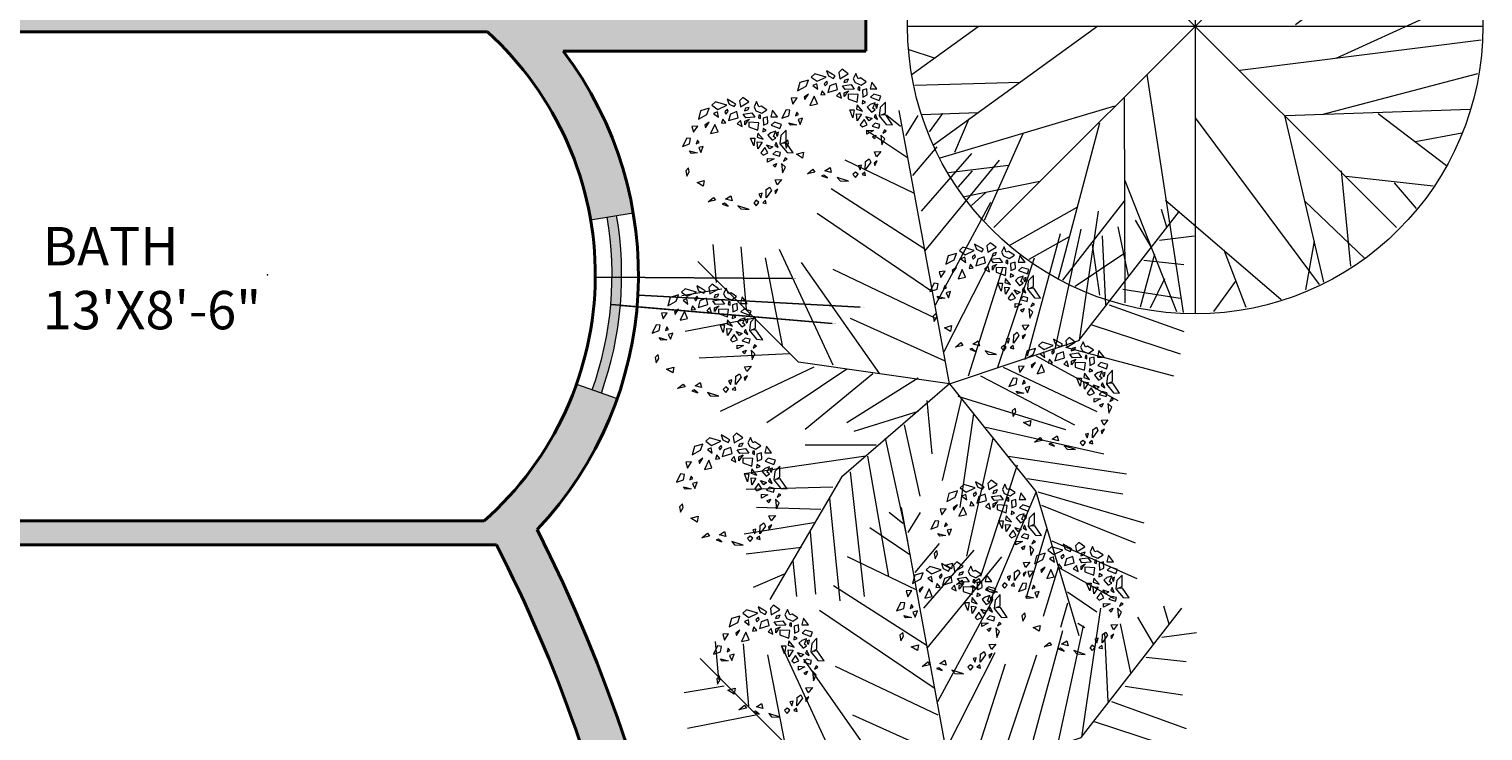
# Model space of a CAD drawing. Units: inches. Extents: x 2330 to 3943, y 1763 to 3461.
# Tile 30 of 40: x 3281 to 3584, y 2829 to 2975. Entities that reach past the tile are written whole.
import ezdxf

# ---------------------------------------------------------------- set-up
doc = ezdxf.new("R2010")
doc.units = ezdxf.units.IN
for name, color, linetype, lineweight in [('A-ANNO-DIMS', 2, 'Continuous', 18), ('A-AREA-IDEN', 7, 'Continuous', 18), ('A-GLAZ', 4, 'Continuous', 18), ('A-WALL', 7, 'Continuous', 40), ('A-WALL-PATT', 252, 'Continuous', 13), ('L-PLNT', 94, 'Continuous', 13)]:
    doc.layers.add(name, color=color, linetype=linetype, lineweight=lineweight)
doc.styles.get("Standard").update_dxf_attribs({"font": 'arial.ttf'})
doc.dimstyles.get("Standard").update_dxf_attribs({"dimtxt": 0.18, "dimasz": 0.18, "dimexe": 0.18, "dimexo": 0.0625, "dimgap": 0.09, "dimtad": 0, "dimtih": 1, "dimtoh": 1, "dimdec": 4, "dimzin": 0, "dimdsep": 46, "dimtxsty": 'Standard', "dimcen": 0.09, "dimadec": 0, "dimazin": 0, "dimtfac": 1, "dimtdec": 4, "dimtofl": 0, "dimtmove": 0, "dimatfit": 3, "dimfxl": 1, "dimtolj": 1, "dimtzin": 0, "dimarcsym": 0})

# ---------------------------------------------------------------- blocks, each defined once
blk = doc.blocks.new('*U12')
for p, q in [((-10.186, 53.64), (-13.084, 55.962)), ((0, 0), (-10.5, 57)), ((-9.099, 51.782), (-6.563, 55.962)), ((-8.737, 47.138), (-17.069, 52.711)), ((-7.65, 43.423), (-2.578, 49.46)), ((-7.288, 39.707), (-21.778, 46.673)), ((-5.839, 35.992), (4.667, 48.067)), ((-5.114, 27.632), (10.463, 46.673)), ((-5.114, 28.097), (-24.676, 40.636)), ((-2.941, 16.486), (8.652, 37.85)), ((44.153, 36.456), (45.239, 32.741)), ((-3.665, 19.273), (-27.574, 35.527)), ((27, 9), (48, 36)), ((27.127, 9.056), (31.112, 35.992)), ((38.719, 34.134), (41.979, 28.561)), ((16.259, 5.805), (23.142, 31.348)), ((22.055, 7.198), (27.489, 32.277)), ((31.836, 30.883), (32.561, 16.486)), ((35.096, 32.741), (37.27, 22.524)), ((43.791, 29.954), (51.036, 30.883)), ((-48.585, 21.131), (-49.309, 29.026)), ((-43.513, 28.561), (-42.427, 15.558)), ((-35.544, 28.097), (-24.314, 3.947)), ((-31.5, 4.5), (-52.5, 25.5)), ((-38.442, 26.239), (-34.819, 7.663)), ((-14.533, 2.09), (-30.834, 25.31)), ((-1.129, 6.734), (9.014, 26.704)), ((3.942, 1.625), (11.187, 24.381)), ((10.101, 3.483), (17.708, 26.239)), ((40.53, 25.775), (48.862, 24.846)), ((-24.314, 23.917), (-2.941, 13.7)), ((-47.498, 19.737), (-55.83, 18.344)), ((36.183, 19.737), (48.137, 17.88)), ((33.285, 16.486), (48.862, 10.913)), ((-40.615, 13.7), (-55.105, 10.913)), ((-20.691, 13.7), (-1.129, 4.876)), ((29.662, 12.307), (48.137, 6.269)), ((-33.37, 6.269), (-52.207, 5.34)), ((0, 0), (27, 9)), ((24.229, 7.663), (46.688, 1.625)), ((-28.299, 3.483), (-47.86, -5.805)), ((0, 0), (-31.5, 4.5)), ((11.187, 3.483), (30.749, -5.805)), ((18.07, 5.805), (35.096, -3.483)), ((-21.416, 3.018), (-38.079, -8.128)), ((-15.982, 2.09), (-30.11, -9.521)), ((0, 0), (-22.5, -19.5)), ((-6.563, 1.161), (-21.416, -8.128)), ((0, 0), (18, -22.5)), ((6.478, 1.625), (26.04, -8.592)), ((2.493, -3.019), (-1.491, -20.202)), ((1.769, -2.555), (24.229, -9.521)), ((-6.563, -5.805), (-19.967, -9.985)), ((-4.752, -3.483), (-3.665, -14.629)), ((-9.461, -8.592), (-6.201, -23.453)), ((5.029, -6.27), (2.131, -25.775)), ((7.565, -9.056), (32.198, -14.629)), ((-13.446, -11.378), (-8.737, -32.741)), ((9.014, -11.378), (3.58, -35.992)), ((-17.431, -15.094), (-42.789, -18.809)), ((-15.257, -12.772), (-30.11, -12.772)), ((-17.069, -15.094), (-12.721, -40.172)), ((12.274, -15.094), (36.907, -18.809)), ((14.085, -16.951), (6.478, -40.172)), ((-22.5, -19.5), (-37.5, -45)), ((-20.691, -18.345), (-17.793, -44.352)), ((16.259, -19.738), (36.183, -22.989)), ((-24.314, -21.596), (-42.427, -22.06)), ((-25.038, -23.918), (-22.865, -45.281)), ((18.07, -22.524), (8.289, -45.745)), ((18, -22.5), (27, -52.5)), ((18.433, -22.524), (40.53, -29.026)), ((-26.849, -26.24), (-40.253, -25.775)), ((19.157, -25.311), (38.719, -33.206)), ((-28.299, -29.026), (-42.789, -31.348)), ((-29.023, -30.884), (-27.936, -43.887)), ((20.244, -30.419), (15.897, -44.816)), ((21.331, -32.741), (39.081, -40.636)), ((-30.834, -34.135), (-42.427, -35.528)), ((-32.646, -36.921), (-31.921, -44.352)), ((22.78, -37.85), (19.519, -48.532)), ((22.78, -38.314), (34.372, -44.816)), ((-34.457, -39.708), (-40.978, -42.494)), ((24.591, -43.423), (30.749, -47.603)), ((24.591, -45.745), (23.142, -50.854)), ((26.764, -49.925), (28.213, -50.854))]:
    blk.add_line(p, q)
blk = doc.blocks.new('*U13')
for points in [[(-5.78, 9.75), (-7.54, 9.23), (-8.01, 7.5), (-6.26, 8.45)], [(-4.43, 11.05), (-5.18, 10.36), (-3.96, 9.49), (-2.07, 10.36)], [(-1.94, 9.49), (-2.48, 8.97), (-2.27, 8.54), (-1.8, 9.06)], [(-2, 11.66), (-1.6, 10.62), (-0.52, 10.1), (-0.18, 10.62), (-0.79, 10.96)], [(1.24, 12), (0.56, 11.31), (0.76, 10.01), (2.52, 11.05)], [(2.59, 9.93), (1.84, 9.75), (1.64, 9.23), (2.32, 9.41)], [(4.14, 11.14), (3.6, 10.01), (4, 9.23), (5.22, 8.71), (6.3, 9.41), (5.08, 10.19), (4.61, 10.01)], [(7.45, 9.32), (7.11, 7.94), (8.52, 7.94)], [(-5.78, 6.81), (-6.66, 6.21), (-6.52, 5.69)], [(-4.57, 6.38), (-5.45, 4.47), (-3.89, 4.82)], [(-4.84, 8.63), (-3.83, 7.85), (-4.03, 8.97)], [(-2.88, 7.5), (-3.15, 6.64), (-2.27, 6.72)], [(0.02, 9.06), (-1.33, 8.54), (-1.73, 7.16), (0.29, 7.76)], [(0.76, 7.16), (0.09, 6.46), (1.1, 5.95)], [(1.37, 8.54), (3.13, 8.8), (3.8, 7.85), (1.91, 7.76)], [(1.71, 6.29), (1.71, 7.07), (2.65, 7.5), (2.11, 6.9)], [(2.52, 6.81), (2.52, 5.86), (4.41, 5.17), (4.61, 6.72)], [(4.61, 8.28), (4.54, 7.76), (4.95, 7.59), (4.95, 8.28)], [(6.43, 7.94), (5.49, 7.68), (5.56, 6.21), (6.5, 6.64)], [(7.85, 6.81), (7.18, 6.21), (9, 5.51), (9.33, 6.38)], [(-11.32, 1.79), (-9.83, 2.31), (-9.63, 3.44), (-10.44, 3.52)], [(-8.14, 6.03), (-9.36, 5.95), (-9.02, 4.73)], [(-8.21, 3.09), (-8.48, 2.31), (-7.87, 2.57)], [(3.53, 1.88), (2.86, 3.52), (3.8, 3.52)], [(4.41, 4.56), (4.27, 3.7), (5.49, 3.26)], [(5.49, 5.51), (5.42, 4.82), (6.16, 5.08)], [(8.12, 4.99), (7.11, 4.65), (6.5, 4.13), (7.38, 3.09), (8.12, 3.52), (7.65, 3.87)], [(8.73, 4.73), (8.19, 4.56), (8.39, 3.87), (8.59, 4.04)], [(10.28, 5.17), (9.2, 4.04), (9, 2.31), (10.48, 0.49), (11.76, 0.41), (10.35, 2.48), (9.33, 2.4), (10.28, 2.83)], [(-8.21, 0.41), (-9.43, 0.32), (-9.83, 0.84)], [(-7, 1.79), (-7.94, 1.53), (-7.47, 0.49)], [(4.27, 2.74), (5.29, 2.66), (4.41, 1.27)], [(5.83, 1.53), (5.02, 0.41), (5.49, -0.02), (6.5, 0.41)], [(7.51, 1.71), (6.91, 1.27), (6.23, 2.14)], [(8.12, 0.75), (7.51, 0.15), (8.93, -0.28), (9.13, 0.49)], [(8.19, 2.57), (7.92, 2.05), (8.66, 1.53)], [(-10.03, -2.71), (-10.64, -3.31), (-10.44, -4.44), (-9.9, -3.49)], [(7.78, -0.8), (6.43, -1.5), (6.43, -0.72)], [(8.32, -1.75), (7.98, -2.53), (7.58, -2.1)], [(9.33, -1.75), (9.54, -3.74), (10.14, -2.53)], [(10.08, -0.63), (9.74, -1.32), (10.48, -0.89)], [(-8.28, -5.73), (-6.79, -5.3), (-7, -6.51)], [(9.33, -5.13), (8.46, -6.25), (7.98, -5.22)], [(-4.84, -8.85), (-4.43, -9.45), (-5.99, -9.8)], [(-2.34, -9.2), (-1.26, -8.5), (-0.99, -9.54)], [(5.29, -7.98), (4.61, -8.16), (5.02, -8.94)], [(6.1, -8.94), (6.16, -7.21), (6.91, -6.69), (7.24, -7.38)], [(8.05, -8.07), (8.59, -7.12), (7.92, -7.55)], [(-2.54, -10.06), (-3.02, -10.23), (-1.8, -10.67)], [(0.22, -10.58), (0.83, -11.27), (2.59, -11.36)], [(4.07, -9.45), (3.53, -9.97), (4.07, -10.58), (4.61, -9.89)], [(6.03, -9.45), (5.42, -9.97), (6.16, -10.15)]]:
    blk.add_lwpolyline(points, close=True)
blk = doc.blocks.new('*U14')
for p, q in [((-22.0458, 42.0753), (-16.5881, 57.6486)), ((-12.5388, 54.9406), (-7.9613, 59.4546)), ((-12.3627, 32.1443), (-12.5388, 58.7776)), ((-5.3205, 59.6806), (16.5105, 16.7963)), ((2.426, 54.9406), (-1.4472, 59.9056)), ((0, 59.9996), (0, -60)), ((0.4894, 48.6208), (3.6584, 59.6806)), ((18.2711, 35.5298), (5.419, 59.6806)), ((9.8203, 51.5549), (12.8133, 58.5516)), ((19.6795, 19.5047), (16.3344, 57.6486)), ((-21.1656, 55.8436), (-0.0388, 45.0094)), ((17.0387, 51.1035), (23.2006, 55.1666)), ((-26.4472, 46.5894), (-26.2712, 53.8116)), ((17.7429, 43.6552), (25.4894, 54.2636)), ((-32.6092, 50.4264), (-23.2782, 23.5674)), ((-31.2008, 51.1035), (-0.2149, 20.1818)), ((31.6513, 50.8778), (30.2429, 30.5643)), ((-37.0107, 47.0408), (-35.25, 35.5298)), ((31.1232, 42.5267), (35.8767, 48.1693)), ((-40.1797, 44.558), (-36.4825, 43.2038)), ((-43.8768, 36.4326), (-44.405, 40.2696)), ((42, 42), (-42, -42)), ((42, -42), (-42, 42)), ((-45.8134, 38.2383), (-40.5318, 33.0471)), ((37.1091, 37.1098), (46.6161, 37.5612)), ((36.2288, 25.1474), (48.9049, 35.0784)), ((-49.8627, 32.8214), (-32.7853, 32.8214)), ((-53.2078, 27.4044), (-40.1797, 20.859)), ((23.3767, 23.3417), (53.3063, 27.4044)), ((-54.7923, 24.4702), (-47.75, 21.0847)), ((54.3626, 25.3731), (20.9119, 0.3198)), ((-32.2571, 20.6333), (-59.1937, 9.348)), ((-56.0247, 20.859), (-20.8134, 20.859)), ((-57.081, 17.9248), (-47.0458, 14.7649)), ((-58.6656, 12.7336), (-35.9543, 7.5424)), ((38.5175, 13.4107), (58.2359, 13.6364)), ((-59.7219, 2.8025), (-12.0106, 12.0565)), ((29.3626, -6.6771), (59.4682, 7.091)), ((-54.6162, -24.7335), (-20.2853, 0.0941)), ((-60, 0), (60, 0)), ((-45.2853, -0.1316), (-59.0177, -10.0627)), ((9.2922, -9.1598), (59.6443, -2.8401)), ((-59.7219, -4.8714), (-54.2641, -6.6771)), ((-58.4895, -12.3197), (-36.4825, -11.6426)), ((-10.074, -10.0627), (-2.5036, -59.7178)), ((26.3697, -18.4138), (58.9401, -9.8369)), ((-14.8275, -15.0282), (-14.6515, -57.6865)), ((-57.081, -18.4138), (-45.2853, -17.9624)), ((-52.6797, -18.188), (-55.4966, -22.0251)), ((-53.2078, -27.442), (-16.7641, -16.6081)), ((18.7992, -18.6394), (57.3556, -17.2853)), ((38.1654, -18.188), (52.426, -29.0219)), ((-47.2219, -19.3166), (-50.2148, -26.3135)), ((-19.9331, -20.2194), (-28.5599, -52.721)), ((-0.0388, -19.0909), (25.8415, -53.8495)), ((18.6232, -18.6394), (26.7218, -53.3981)), ((-35.9543, -22.4765), (-44.0529, -40.5329)), ((45.9119, -24.0564), (55.595, -22.2508)), ((-38.9472, -29.0219), (-51.4472, -30.6018)), ((-46.5177, -30.1504), (-49.5106, -33.536)), ((30.419, -30.1504), (32.3556, -50.0125)), ((-32.4331, -32.4075), (-48.1021, -35.5674)), ((-14.6515, -32.1818), (-3.912, -59.4922)), ((31.4753, -31.279), (49.6091, -33.3103)), ((41.5105, -32.6332), (46.088, -38.0501)), ((-43.7008, -34.6645), (-46.6937, -37.373)), ((-14.6515, -36.2445), (-27.6797, -52.9467)), ((-6.2008, -36.2445), (17.919, -57.0094)), ((-24.6867, -37.8244), (-38.7712, -45.7241)), ((22.8485, -36.4702), (35.3485, -48.4326)), ((-26.2712, -43.9185), (-34.7219, -48.6583)), ((24.7852, -44.8213), (23.0246, -54.978)), ((-14.6515, -47.3041), (-25.0388, -54.3009)), ((-21.5177, -45.4984), (-19.9331, -56.1065)), ((-8.4895, -47.5298), (-11.4825, -58.5893)), ((5.9471, -46.6269), (10.5246, -58.5893)), ((-6.3768, -52.721), (-9.3698, -58.815)), ((8.4119, -53.1724), (3.8344, -59.4922))]:
    blk.add_line(p, q)
blk.add_circle((0, 0), 60)
blk = doc.blocks.new('*D99')
at = {"layer": 'A-ANNO-DIMS', "color": 0, "lineweight": -2, "transparency": 16777216}
for p, q in [((3330.82, 2923.97), (3331, 2923.97)), ((3330.91, 2923.88), (3330.91, 2924.06)), ((3454.5, 2917.21), (3408.33, 2919.74))]:
    blk.add_line(p, q, dxfattribs=at)
at = {"layer": 'A-ANNO-DIMS', "color": 0, "transparency": 16777216}
blk.add_solid([(3408.34, 2919.77), (3408.33, 2919.71), (3408.15, 2919.75)], dxfattribs=at)
at = {"layer": 'Defpoints', "color": 0, "transparency": 16777216}
for p in [(3330.91, 2923.97), (3408.15, 2919.75)]:
    blk.add_point(p, dxfattribs=at)
at = {"layer": 'A-ANNO-DIMS', "color": 0, "transparency": 16777216, "insert": (3454.98, 2917.21), "char_height": 0.18, "attachment_point": 5}
blk.add_mtext('\\A1;R77.36', dxfattribs=at)
blk = doc.blocks.new('*D100')
at = {"layer": 'A-ANNO-DIMS', "color": 0, "lineweight": -2, "transparency": 16777216}
for p, q in [((3330.82, 2923.97), (3331, 2923.97)), ((3330.91, 2923.88), (3330.91, 2924.06)), ((3448.65, 2913.83), (3404.68, 2917.61))]:
    blk.add_line(p, q, dxfattribs=at)
at = {"layer": 'A-ANNO-DIMS', "color": 0, "transparency": 16777216}
blk.add_solid([(3404.68, 2917.64), (3404.67, 2917.58), (3404.5, 2917.63)], dxfattribs=at)
at = {"layer": 'Defpoints', "color": 0, "transparency": 16777216}
for p in [(3330.91, 2923.97), (3404.5, 2917.63)]:
    blk.add_point(p, dxfattribs=at)
at = {"layer": 'A-ANNO-DIMS', "color": 0, "transparency": 16777216, "insert": (3449.13, 2913.83), "char_height": 0.18, "attachment_point": 5}
blk.add_mtext('\\A1;R73.86', dxfattribs=at)
blk = doc.blocks.new('*D101')
at = {"layer": 'A-ANNO-DIMS', "color": 0, "lineweight": -2, "transparency": 16777216}
for p, q in [((3330.82, 2923.97), (3331, 2923.97)), ((3330.91, 2923.88), (3330.91, 2924.06)), ((3445.46, 2914.1), (3402.68, 2917.79))]:
    blk.add_line(p, q, dxfattribs=at)
at = {"layer": 'A-ANNO-DIMS', "color": 0, "transparency": 16777216}
blk.add_solid([(3402.69, 2917.82), (3402.68, 2917.76), (3402.5, 2917.8)], dxfattribs=at)
at = {"layer": 'Defpoints', "color": 0, "transparency": 16777216}
for p in [(3330.91, 2923.97), (3402.5, 2917.8)]:
    blk.add_point(p, dxfattribs=at)
at = {"layer": 'A-ANNO-DIMS', "color": 0, "transparency": 16777216, "insert": (3445.94, 2914.1), "char_height": 0.18, "attachment_point": 5}
blk.add_mtext('\\A1;R71.86', dxfattribs=at)
blk = doc.blocks.new('*D102')
at = {"layer": 'A-ANNO-DIMS', "color": 0, "lineweight": -2, "transparency": 16777216}
for p, q in [((3330.82, 2923.97), (3331, 2923.97)), ((3330.91, 2923.88), (3330.91, 2924.06)), ((3440.28, 2923.21), (3399.45, 2923.49))]:
    blk.add_line(p, q, dxfattribs=at)
at = {"layer": 'A-ANNO-DIMS', "color": 0, "transparency": 16777216}
blk.add_solid([(3399.45, 2923.52), (3399.45, 2923.46), (3399.27, 2923.5)], dxfattribs=at)
at = {"layer": 'Defpoints', "color": 0, "transparency": 16777216}
for p in [(3330.91, 2923.97), (3399.27, 2923.5)]:
    blk.add_point(p, dxfattribs=at)
at = {"layer": 'A-ANNO-DIMS', "color": 0, "transparency": 16777216, "insert": (3440.76, 2923.21), "char_height": 0.18, "attachment_point": 5}
blk.add_mtext('\\A1;R68.36', dxfattribs=at)

msp = doc.modelspace()

# ---------------------------------------------------------------- hatches: boundary and pattern name
at = {"layer": 'A-GLAZ'}
h = msp.add_hatch(color=256, dxfattribs=at)
h.dxf.hatch_style = 1
h.paths.add_polyline_path([(3403.7236, 2936.3476), (3401.7519, 2936.0123, -0.12785783), (3398.6504, 2899.9877), (3400.5358, 2899.3203, 0.12785783)])
at = {"layer": 'A-WALL-PATT'}
h = msp.add_hatch(color=256, dxfattribs=at)
h.dxf.hatch_style = 1
h.paths.add_polyline_path([(3241.6605, 2974.6524), (3376.7746, 2974.6524, -0.16828569), (3398.3014, 2935.4254), (3407.174, 2936.9344, 0.12044914), (3392.5913, 2970.6524), (3455.6605, 2970.6524), (3455.6605, 3018.6524), (3446.6605, 3018.6524), (3446.6605, 2979.6524), (3275.6605, 2979.6524), (3275.6605, 3018.6524), (3270.6605, 3018.6524), (3270.6605, 2979.6524), (3154.6605, 2979.6524), (3154.6605, 2918.1524), (3150.6605, 2918.1524), (3150.6605, 2913.1524), (3154.6605, 2913.1524), (3154.6605, 2863.6524), (3159.6605, 2863.6524), (3159.6605, 2867.6524), (3196.6605, 2867.6524), (3196.6605, 2872.6524), (3159.6605, 2872.6524), (3159.6605, 2974.6524), (3236.6605, 2974.6524), (3236.6605, 2906.6524), (3241.6605, 2906.6524)])
h = msp.add_hatch(color=256, dxfattribs=at)
h.dxf.hatch_style = 1
h.paths.add_polyline_path([(3387.1394, 2870.8379, 0.10459296), (3403.8352, 2898.1524), (3395.3511, 2901.1556, -0.12790871), (3376.0739, 2872.6524), (3241.6605, 2872.6524), (3241.6605, 2876.6524), (3236.6605, 2876.6524), (3236.6605, 2872.6524), (3232.6605, 2872.6524), (3232.6605, 2867.6524), (3378.6605, 2867.6524, -0.07524693), (3407.8539, 2780.6064), (3416.7189, 2782.159, 0.07442358)])

# ---------------------------------------------------------------- linework, layer by layer
at = {"layer": 'A-GLAZ'}
for p, q in [((3398.3014, 2935.4254), (3407.174, 2936.9344)), ((3395.3511, 2901.1556), (3403.8352, 2898.1524))]:
    msp.add_line(p, q, dxfattribs=at)
for radius in [71.855, 73.855]:
    msp.add_arc((3330.914, 2923.9651), radius, 340.507033, 9.65176, dxfattribs=at)
at = {"layer": 'A-WALL'}
for p, q in [((3455.6605, 3162.6524), (3455.6605, 2970.6524)), ((3241.6605, 2974.6524), (3376.7746, 2974.6524)), ((3392.5913, 2970.6524), (3455.6605, 2970.6524)), ((3241.6605, 2872.6524), (3376.0739, 2872.6524)), ((3232.6605, 2867.6524), (3378.6605, 2867.6524))]:
    msp.add_line(p, q, dxfattribs=at)
for centre, radius, start, end in [((3330.914, 2923.9651), 68.355, 311.350834, 47.861979), ((3330.914, 2923.9651), 77.355, 316.622935, 37.124323), ((3105.6935, 2727.6869), 315.7595, 317.571214, 26.95911), ((3105.6935, 2727.6869), 306.7595, 355.880906, 27.146756)]:
    msp.add_arc(centre, radius, start, end, dxfattribs=at)

# ---------------------------------------------------------------- block references
at = {"layer": 'L-PLNT'}
for name, p in [('*U14', (3524.3948, 2975.8319)), ('*U13', (3449.4872, 2954.8527)), ('*U13', (3428.7734, 2948.9828)), ('*U12', (3473.1399, 2901.2527)), ('*U13', (3480.3812, 2918.6863)), ('*U13', (3422.4242, 2910.0354)), ('*U13', (3496.8672, 2898.8899)), ('*U13', (3427.4952, 2878.9199)), ('*U13', (3480.5657, 2869.1674)), ('*U12', (3473.6244, 2818.4657)), ('*U13', (3498.8602, 2856.1639)), ('*U13', (3473.4432, 2852.0945)), ('*U13', (3435.2247, 2843.039))]:
    msp.add_blockref(name, p, dxfattribs=at)

# ---------------------------------------------------------------- texts
at = {"layer": 'A-AREA-IDEN', "insert": (3284.0461, 2933.9492), "char_height": 8, "attachment_point": 1}
msp.add_mtext_dynamic_manual_height_columns('BATH\\P13\'X8\'-6"', width=66.36581, gutter_width=12.5, heights=[0], dxfattribs=at)

# ---------------------------------------------------------------- dimensions: what is measured, and where the dimension line sits
at = {"layer": 'A-ANNO-DIMS'}
for center, mpoint, picture, middle in [((3330.914, 2923.9651), (3408.1539, 2919.746), '*D99', (3454.4978, 2917.2146)), ((3330.914, 2923.9651), (3404.4968, 2917.63), '*D100', (3448.6465, 2913.829)), ((3330.91397, 2923.96508), (3402.5042, 2917.80198), '*D101', (3445.45835, 2914.10412)), ((3330.914, 2923.9651), (3399.2674, 2923.496), '*D102', (3440.2794, 2923.2145))]:
    dim = msp.add_radius_dim(center=center, mpoint=mpoint, dimstyle='Standard', override={"dimdec": 2, "dimlfac": 1, "dimrnd": 0, "dimzin": 0, "dimdsep": 46, "dimlunit": 2}, dxfattribs=at)
    dim.commit()
    dim.dimension.update_dxf_attribs({"geometry": picture, "text_midpoint": middle, "dimtype": 164})

doc.saveas('drawing.dxf')
